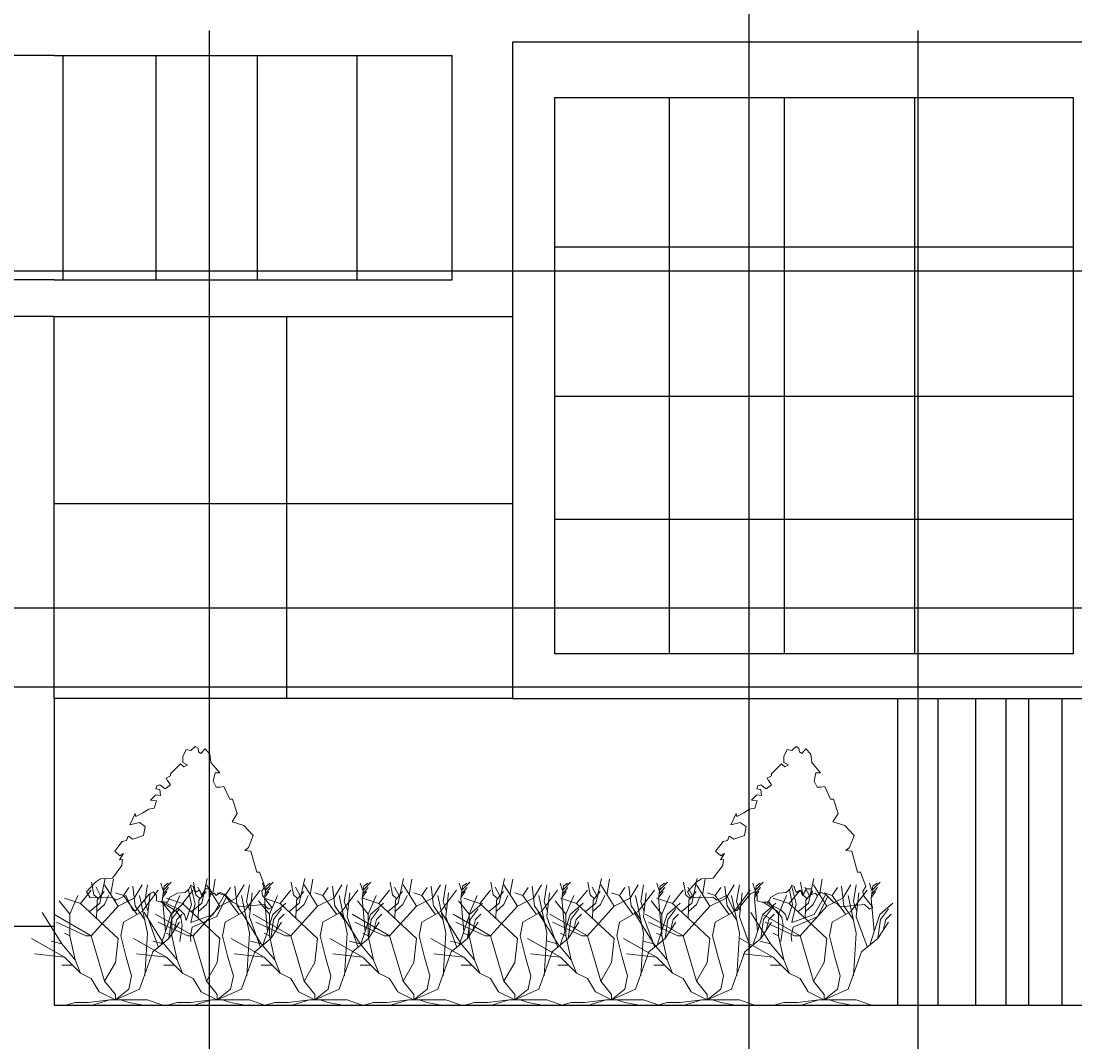
# Model space of a CAD drawing. Units: inches. Extents: x -117 to 121, y -77 to 40.
# Tile 22 of 45: x 3 to 28, y -32 to -8. Entities that reach past the tile are written whole.
import ezdxf

# ---------------------------------------------------------------- set-up
doc = ezdxf.new("R2010")
doc.units = ezdxf.units.IN
doc.header["$MEASUREMENT"] = 0
for name, color, linetype, lineweight in [('A-ANNO-DIMS', 2, 'Continuous', 18), ('A-ELEV', 7, 'Continuous', 25), ('L-PLNT', 3, 'Continuous', 13)]:
    doc.layers.add(name, color=color, linetype=linetype, lineweight=lineweight)
doc.styles.get("Standard").update_dxf_attribs({"font": 'arial.ttf'})
doc.dimstyles.get("Standard").update_dxf_attribs({"dimtxt": 0.18, "dimasz": 0.18, "dimexe": 0.18, "dimexo": 0.0625, "dimgap": 0.09, "dimtad": 0, "dimtih": 1, "dimtoh": 1, "dimdec": 4, "dimzin": 0, "dimdsep": 46, "dimtxsty": 'Standard', "dimcen": 0.09, "dimadec": 0, "dimazin": 0, "dimtfac": 1, "dimtdec": 4, "dimtofl": 0, "dimtmove": 0, "dimatfit": 3, "dimfxl": 1, "dimtolj": 1, "dimtzin": 0, "dimarcsym": 0})

# ---------------------------------------------------------------- blocks, each defined once
blk = doc.blocks.new('*U3')
for p, q in [((-11.433, 18.289), (-10.457, 22.749)), ((-12.471, 19.775), (-12.898, 22.044)), ((-11.28, 19.619), (-12.104, 21.184)), ((-8.16, 17.76), (-10.56, 21.6)), ((-9.48, 19.775), (-8.992, 22.592)), ((-7.2, 19.68), (-6.24, 21.12)), ((-5.086, 17.741), (-5.513, 21.34)), ((-5.28, 19.2), (-3.84, 21.6)), ((-3.377, 18.602), (-2.888, 21.575)), ((-0.508, 21.888), (-0.081, 20.558)), ((-0.203, 19.149), (0.102, 21.34)), ((-0.02, 20.01), (0.896, 21.105)), ((0.041, 20.714), (1.384, 22.044)), ((0.102, 21.34), (0.835, 21.888)), ((-14.88, 18.24), (-17.76, 19.2)), ((-16.8, 16.32), (-15.36, 19.68)), ((-14.88, 18.24), (-12.96, 20.64)), ((-11.677, 19.071), (-12.471, 19.775)), ((-11.921, 18.836), (-10.64, 20.401)), ((-10.579, 18.054), (-9.846, 19.697)), ((-7.2, 19.68), (-8.64, 20.16)), ((-8.16, 17.76), (-5.28, 19.2)), ((-4.8, 16.32), (-7.2, 19.68)), ((-2.88, 12.96), (-4.32, 19.68)), ((-3.84, 16.8), (-0.96, 20.64)), ((-2.88, 15.84), (-2.4, 20.16)), ((0.346, 13.203), (-0.203, 19.149)), ((-0.142, 19.384), (0.59, 20.401)), ((-16.8, 16.32), (-18.72, 18.72)), ((-8.16, 12), (-14.88, 18.24)), ((-13.325, 16.724), (-11.433, 18.289)), ((-12.96, 12.48), (-8.16, 17.76)), ((-12.043, 15.628), (-11.921, 18.836)), ((-11.982, 16.802), (-10.579, 18.054)), ((-3.377, 15.315), (-5.086, 17.819)), ((-2.766, 16.802), (-3.377, 18.602)), ((1.323, 16.254), (3.642, 18.289)), ((1.44, 15.36), (2.88, 17.28)), ((-18.24, 11.04), (-21.755, 16.655)), ((-12.96, 12.48), (-19.68, 16.32)), ((-16.8, 12.48), (-16.8, 16.32)), ((-7.2, 14.88), (-3.84, 16.8)), ((-0.96, 10.56), (-2.88, 15.84)), ((0.346, 13.203), (1.323, 16.254)), ((0.96, 12), (1.44, 15.36)), ((1.92, 13.44), (2.4, 15.36)), ((2.4, 15.36), (3.36, 16.32)), ((-13.92, 12.48), (-19.2, 14.88)), ((-7.68, 12.48), (-7.2, 14.88)), ((0.96, 12), (2.88, 14.88)), ((-17.76, 8.64), (-23.663, 11.961)), ((-18.24, 11.04), (-20.16, 11.52)), ((-16.8, 12.48), (-17.76, 12.96)), ((-15.84, 8.16), (-16.8, 12.48)), ((-12.96, 12.48), (-13.92, 12.48)), ((-10.56, 4.32), (-12.96, 12.48)), ((-8.64, 7.68), (-8.16, 12)), ((-6.72, 8.64), (-7.68, 12.48)), ((-3.36, 5.28), (-2.88, 12.96)), ((-1.92, 9.6), (0.96, 12)), ((-0.48, 10.8), (0.346, 13.203)), ((-15.84, 8.16), (-18.24, 11.04)), ((-4.32, 2.88), (-1.92, 9.6)), ((-17.76, 8.64), (-23.128, 9.222)), ((-14.88, 5.76), (-17.76, 8.64)), ((-14.88, 5.76), (-15.84, 8.16)), ((-10.56, 4.32), (-8.64, 7.68)), ((-5.76, 5.28), (-6.72, 8.64)), ((-16.32, 7.2), (-18.24, 7.2)), ((-12.96, 4.8), (-14.88, 5.76)), ((-11.52, 2.4), (-12.96, 4.8)), ((-8.64, 1.92), (-10.56, 4.32)), ((-6.24, 2.88), (-5.76, 5.28)), ((-8.64, 0.96), (-11.52, 2.4)), ((-8.64, 0.96), (-4.32, 2.88)), ((-8.64, 0.96), (-6.24, 2.88)), ((-8.64, 0.96), (-8.64, 1.92)), ((-15.84, 0.48), (-17.76, 0)), ((-13.44, 0.48), (-15.84, 0.48)), ((-9.6, 0.96), (-13.44, 0.48)), ((-9.6, 0.96), (-12.96, 0)), ((-9.6, 0.96), (-7.68, 0.96)), ((-8.64, 0.96), (-2.88, 0.96)), ((-7.68, 0.96), (-6.24, 0.48)), ((-6.24, 0.48), (-3.36, 0)), ((-2.88, 0.96), (0, 0))]:
    blk.add_line(p, q)
blk = doc.blocks.new('*U4')
for points in [[(22.0124, 137.721), (18.5475, 141.5624), (15.5282, 138.2446), (13.8028, 139.3505), (13.3714, 142.1153), (11.2148, 143.2214), (8.1954, 140.4564), (4.7447, 141.0094), (2.1567, 136.0326), (2.1567, 131.6088), (5.6074, 129.9499), (3.0193, 128.2909), (0.4313, 130.5029), (-6.9015, 123.3141), (-6.9015, 121.6552), (-9.9208, 119.9963), (-9.0581, 118.3373), (-6.9015, 115.0195), (-10.7835, 112.2546), (-14.6656, 115.0195), (-16.8222, 114.4665), (-17.6849, 112.2546), (-14.6656, 111.7016), (-14.2342, 107.2778), (-17.6065, 107.8307), (-21.5669, 103.9599), (-17.2536, 103.4069), (-18.9789, 97.8771), (-22.8609, 97.3241), (-27.1743, 94.5593), (-32.3504, 91.7944), (-32.7817, 94.0063), (-36.6638, 85.7116), (-29.7624, 87.3705), (-25.449, 84.6056), (-26.743, 77.9699), (-34.507, 75.205), (-37.9578, 77.4169), (-39.2518, 74.099), (-42.2711, 73.5461), (-44.8592, 70.2282), (-47.8786, 66.3574), (-43.9965, 63.0395), (-41.4085, 64.6985), (-44.3346, 59.8898), (-42.2089, 60.1377), (-42.5159, 55.7849), (-49.6039, 46.4502), (-58.2307, 45.8972), (-62.1127, 43.6853), (-68.5828, 36.4966), (-65.9947, 32.0727), (-50.0352, 32.6257), (-47.0159, 30.4138), (-39.6831, 33.7317), (-34.507, 22.6721), (-32.3504, 22.6721), (-22.4296, 34.8376), (-19.4102, 36.4966), (-17.2536, 33.7317), (-17.2536, 29.8608), (-13.8028, 28.7549), (-9.0581, 28.7549), (-7.3328, 32.6257), (-1.7254, 35.3906), (3.8821, 35.9436), (6.4701, 38.1555), (6.9014, 38.7085), (8.1954, 41.4734), (9.9208, 40.3674), (11.2148, 35.9436), (14.2341, 37.6025), (15.0968, 36.4966), (15.9595, 33.7317), (18.9789, 38.7085), (21.9982, 38.7085), (23.2922, 36.4966), (21.9982, 34.2847), (25.4489, 35.3906), (26.743, 33.7317), (29.7623, 35.9436), (32.7817, 34.8376), (38.8204, 28.7549), (41.4084, 27.6489), (43.5651, 25.437), (61.6813, 27.0959), (65.132, 23.7781), (67.7201, 24.884), (60.8186, 33.7317), (60.3873, 37.0495), (62.544, 40.3674), (58.662, 50.874), (56.5053, 50.874), (52.1919, 66.3574), (47.8785, 66.9103), (50.4665, 69.1222), (53.9172, 77.9699), (47.0158, 85.1586), (38.3891, 87.9235), (42.2711, 94.0063)], [(42.2711, 94.0063), (38.8204, 104.5129), (36.6637, 104.5129), (32.3503, 113.9135), (29.7623, 113.3605), (26.743, 113.3605), (24.5862, 117.7844), (25.8802, 123.8671), (29.331, 123.8671), (22.8609, 131.6088), (21.9982, 137.6916)], [(8.1954, 40.3674), (11.2148, 27.6489), (8.1954, 13.8245), (24.5862, 19.9072), (32.7817, 34.2847)], [(-9.9208, 28.2019), (0, 23.2251), (3.4507, 19.9072), (4.7447, 15.4834), (8.6267, 27.0959), (6.4701, 37.6025)], [(34.5071, 33.1787), (27.1743, 18.2483), (9.0581, 10.5066), (7.7641, 3.8708), (8.1954, 0)], [(-12.9401, 28.7549), (-2.588, 22.1191), (0.8626, 17.6953), (1.7253, 11.6125), (0, 0)]]:
    blk.add_lwpolyline(points)
blk = doc.blocks.new('*D32')
at = {"layer": 'A-ANNO-DIMS', "color": 0, "lineweight": -2, "transparency": 16777216}
for p, q in [((-3.85, -45.55), (-3.85, 38.61)), ((20.293, -45.55), (20.293, 38.61)), ((-3.67, 38.43), (7.757, 38.43)), ((20.113, 38.43), (8.686, 38.43))]:
    blk.add_line(p, q, dxfattribs=at)
at = {"layer": 'A-ANNO-DIMS', "color": 0, "transparency": 16777216}
for points in [[(-3.67, 38.46), (-3.67, 38.4), (-3.85, 38.43)], [(20.113, 38.46), (20.113, 38.4), (20.293, 38.43)]]:
    blk.add_solid(points, dxfattribs=at)
at = {"layer": 'Defpoints', "color": 0, "transparency": 16777216}
for p in [(20.293, 38.43), (-3.85, -45.613), (20.293, -45.613)]:
    blk.add_point(p, dxfattribs=at)
at = {"layer": 'A-ANNO-DIMS', "color": 0, "transparency": 16777216, "insert": (8.222, 38.43), "char_height": 0.18, "attachment_point": 5}
blk.add_mtext('\\A1;24.142', dxfattribs=at)
blk = doc.blocks.new('*D49')
at = {"layer": 'A-ANNO-DIMS', "color": 0, "lineweight": -2, "transparency": 16777216}
for p, q in [((-45.422, -23.501), (120.84, -23.501)), ((120.66, -23.681), (120.66, -31.426)), ((120.66, -39.536), (120.66, -31.79)), ((-45.471, -39.716), (120.84, -39.716))]:
    blk.add_line(p, q, dxfattribs=at)
at = {"layer": 'A-ANNO-DIMS', "color": 0, "transparency": 16777216}
for points in [[(120.63, -23.681), (120.69, -23.681), (120.66, -23.501)], [(120.63, -39.536), (120.69, -39.536), (120.66, -39.716)]]:
    blk.add_solid(points, dxfattribs=at)
at = {"layer": 'Defpoints', "color": 0, "transparency": 16777216}
for p in [(-45.485, -23.501), (120.66, -23.501), (-45.533, -39.716)]:
    blk.add_point(p, dxfattribs=at)
at = {"layer": 'A-ANNO-DIMS', "color": 0, "transparency": 16777216, "insert": (120.66, -31.608), "char_height": 0.18, "attachment_point": 5}
blk.add_mtext('\\A1;16.215', dxfattribs=at)
blk = doc.blocks.new('*D50')
at = {"layer": 'A-ANNO-DIMS', "color": 0, "lineweight": -2, "transparency": 16777216}
for p, q in [((-47.458, -13.74), (120.84, -13.74)), ((120.66, -13.92), (120.66, -17.512)), ((120.66, -21.468), (120.66, -17.876)), ((-47.458, -21.648), (120.84, -21.648))]:
    blk.add_line(p, q, dxfattribs=at)
at = {"layer": 'A-ANNO-DIMS', "color": 0, "transparency": 16777216}
for points in [[(120.63, -13.92), (120.69, -13.92), (120.66, -13.74)], [(120.63, -21.468), (120.69, -21.468), (120.66, -21.648)]]:
    blk.add_solid(points, dxfattribs=at)
at = {"layer": 'Defpoints', "color": 0, "transparency": 16777216}
for p in [(-47.521, -13.74), (120.66, -13.74), (-47.521, -21.648)]:
    blk.add_point(p, dxfattribs=at)
at = {"layer": 'A-ANNO-DIMS', "color": 0, "transparency": 16777216, "insert": (120.66, -17.694), "char_height": 0.18, "attachment_point": 5}
blk.add_mtext('\\A1;7.908', dxfattribs=at)
blk = doc.blocks.new('*D56')
at = {"layer": 'A-ANNO-DIMS', "color": 0, "lineweight": -2, "transparency": 16777216}
for p, q in [((-14.23, -7.853), (-14.23, -77.193)), ((7.628, -8.105), (7.628, -77.193)), ((-14.05, -77.013), (-3.766, -77.013)), ((7.448, -77.013), (-2.835, -77.013))]:
    blk.add_line(p, q, dxfattribs=at)
at = {"layer": 'A-ANNO-DIMS', "color": 0, "transparency": 16777216}
for points in [[(-14.05, -76.983), (-14.05, -77.043), (-14.23, -77.013)], [(7.448, -76.983), (7.448, -77.043), (7.628, -77.013)]]:
    blk.add_solid(points, dxfattribs=at)
at = {"layer": 'Defpoints', "color": 0, "transparency": 16777216}
for p in [(-14.23, -7.791), (7.628, -8.042), (7.628, -77.013)]:
    blk.add_point(p, dxfattribs=at)
at = {"layer": 'A-ANNO-DIMS', "color": 0, "transparency": 16777216, "insert": (-3.301, -77.013), "char_height": 0.18, "attachment_point": 5}
blk.add_mtext('\\A1;21.858', dxfattribs=at)
blk = doc.blocks.new('*D57')
at = {"layer": 'A-ANNO-DIMS', "color": 0, "lineweight": -2, "transparency": 16777216}
for p, q in [((7.628, -8.105), (7.628, -77.193)), ((24.248, -8.105), (24.248, -77.193)), ((7.808, -77.013), (15.483, -77.013)), ((24.068, -77.013), (16.393, -77.013))]:
    blk.add_line(p, q, dxfattribs=at)
at = {"layer": 'A-ANNO-DIMS', "color": 0, "transparency": 16777216}
for points in [[(7.808, -76.983), (7.808, -77.043), (7.628, -77.013)], [(24.068, -76.983), (24.068, -77.043), (24.248, -77.013)]]:
    blk.add_solid(points, dxfattribs=at)
at = {"layer": 'Defpoints', "color": 0, "transparency": 16777216}
for p in [(7.628, -8.042), (24.248, -8.042), (24.248, -77.013)]:
    blk.add_point(p, dxfattribs=at)
at = {"layer": 'A-ANNO-DIMS', "color": 0, "transparency": 16777216, "insert": (15.938, -77.013), "char_height": 0.18, "attachment_point": 5}
blk.add_mtext('\\A1;16.620', dxfattribs=at)
blk = doc.blocks.new('*D58')
at = {"layer": 'A-ANNO-DIMS', "color": 0, "lineweight": -2, "transparency": 16777216}
for p, q in [((24.248, -8.105), (24.248, -77.193)), ((57.61, -7.947), (57.61, -77.193)), ((24.428, -77.013), (40.467, -77.013)), ((57.43, -77.013), (41.392, -77.013))]:
    blk.add_line(p, q, dxfattribs=at)
at = {"layer": 'A-ANNO-DIMS', "color": 0, "transparency": 16777216}
for points in [[(24.428, -76.983), (24.428, -77.043), (24.248, -77.013)], [(57.43, -76.983), (57.43, -77.043), (57.61, -77.013)]]:
    blk.add_solid(points, dxfattribs=at)
at = {"layer": 'Defpoints', "color": 0, "transparency": 16777216}
for p in [(57.61, -7.885), (24.248, -8.042), (57.61, -77.013)]:
    blk.add_point(p, dxfattribs=at)
at = {"layer": 'A-ANNO-DIMS', "color": 0, "transparency": 16777216, "insert": (40.929, -77.013), "char_height": 0.18, "attachment_point": 5}
blk.add_mtext('\\A1;33.362', dxfattribs=at)

msp = doc.modelspace()

# ---------------------------------------------------------------- linework, layer by layer
at = {"layer": 'A-ELEV'}
for p, q in [((29.012, -8.3785), (14.7397, -8.3785)), ((14.7397, -8.3785), (14.7397, -8.8134)), ((3.9947, -8.6912), (-13.7272, -8.6912)), ((3.9947, -8.6912), (13.3263, -8.6912)), ((4.2039, -13.9556), (4.2039, -8.6912)), ((6.3832, -13.9556), (6.3832, -8.6912)), ((8.7651, -13.9556), (8.7651, -8.6912)), ((11.0964, -13.9556), (11.0964, -8.6912)), ((13.3263, -13.9556), (13.3263, -8.6912)), ((14.7397, -8.8134), (14.7397, -23.7756)), ((15.7326, -9.6801), (27.8856, -9.6801)), ((15.7326, -22.7278), (15.7326, -9.6801)), ((18.419, -9.6801), (18.419, -22.7278)), ((21.1133, -9.6801), (21.1133, -22.7278)), ((24.1718, -9.6801), (24.1718, -22.7278)), ((27.8856, -9.6801), (27.8856, -22.7278)), ((15.7326, -13.1807), (27.8856, -13.1807)), ((3.9947, -13.9556), (-13.7272, -13.9556)), ((3.9947, -13.9556), (13.3263, -13.9556)), ((3.9947, -14.8161), (-13.7272, -14.8161)), ((3.9947, -23.7756), (3.9947, -14.8161)), ((3.9947, -14.8161), (14.7397, -14.8161)), ((9.4524, -23.7756), (9.4524, -14.8161)), ((15.7326, -16.6813), (27.8856, -16.6813)), ((3.9947, -19.2007), (14.7397, -19.2007)), ((15.7326, -19.5699), (27.8856, -19.5699)), ((27.8856, -22.7278), (15.7326, -22.7278)), ((22.0645, -22.7074), (22.0645, -22.7278)), ((22.8894, -22.7074), (22.8894, -22.7278)), ((23.7732, -22.7074), (23.7732, -22.7278)), ((24.7159, -22.7074), (24.7159, -22.7278)), ((25.5997, -22.7074), (25.5997, -22.7278)), ((26.312, -22.7074), (26.312, -22.7278)), ((26.8414, -22.7074), (26.8414, -22.7278)), ((27.6241, -22.7074), (27.6241, -22.7278)), ((14.7397, -23.7756), (3.9947, -23.7756)), ((3.9947, -23.7756), (3.9947, -30.968)), ((14.7397, -23.7756), (29.012, -23.7756)), ((23.7732, -23.7756), (23.7732, -30.968)), ((24.7159, -23.7756), (24.7159, -30.968)), ((25.5997, -23.7756), (25.5997, -30.968)), ((26.312, -23.7756), (26.312, -30.968)), ((26.8414, -23.7756), (26.8414, -30.968)), ((27.6241, -23.7756), (27.6241, -30.968)), ((-13.7272, -29.1126), (3.9947, -29.1126)), ((3.9947, -30.968), (21.9795, -30.968)), ((21.9795, -30.968), (38.5013, -30.968))]:
    msp.add_line(p, q, dxfattribs=at)

# ---------------------------------------------------------------- block references
at = {"layer": 'L-PLNT'}
for name, p, xscale, yscale, zscale in [('*U4', (6.9415, -29.4693), 0.0318946538926936, 0.0318946538926936, 0.0318946538926936), ('*U4', (21.0324, -29.4693), 0.0318946538926936, 0.0318946538926936, 0.0318946538926936), ('*U3', (6.5606, -30.9685), 0.1308970629423973, 0.1308970629423973, 0.1308970629423973), ('*U3', (8.9503, -30.9685), 0.1308970629423973, 0.1308970629423973, 0.1308970629423973), ('*U3', (11.2403, -30.9685), 0.1308970629423973, 0.1308970629423973, 0.1308970629423973), ('*U3', (13.5583, -30.9685), 0.1308970629423973, 0.1308970629423973, 0.1308970629423973), ('*U3', (15.924, -30.9685), 0.1308970629423973, 0.1308970629423973, 0.1308970629423973), ('*U3', (18.1942, -30.9685), 0.1308970629423973, 0.1308970629423973, 0.1308970629423973), ('*U3', (20.4405, -30.9685), 0.1308970629423973, 0.1308970629423973, 0.1308970629423973), ('*U3', (23.1804, -30.9685), 0.1308970629423973, 0.1308970629423973, 0.1308970629423973)]:
    msp.add_blockref(name, p, dxfattribs=dict(at, xscale=xscale, yscale=yscale, zscale=zscale))

# ---------------------------------------------------------------- dimensions: what is measured, and where the dimension line sits
at = {"layer": 'A-ANNO-DIMS'}
for base, p1, p2, picture, middle in [((20.2929, 38.4297), (-3.8495, -45.6125), (20.2929, -45.6125), '*D32', (8.2217, 38.4297)), ((7.6284, -77.0135), (-14.2298, -7.7907), (7.6284, -8.0421), '*D56', (-3.3007, -77.0135)), ((57.6104, -77.0135), (24.2481, -8.0421), (57.6104, -7.8846), '*D58', (40.9293, -77.0135)), ((24.2481, -77.0135), (7.6284, -8.0421), (24.2481, -8.0421), '*D57', (15.9383, -77.0135))]:
    dim = msp.add_linear_dim(base=base, p1=p1, p2=p2, dimstyle='Standard', override={"dimdec": 3, "dimlfac": 1, "dimrnd": 0, "dimzin": 0, "dimdsep": 46, "dimlunit": 2}, dxfattribs=at)
    dim.commit()
    dim.dimension.update_dxf_attribs({"geometry": picture, "text_midpoint": middle})
for base, p1, p2, picture, middle in [((120.6602, -13.74), (-47.5206, -21.6476), (-47.5206, -13.74), '*D50', (120.6602, -17.6938)), ((120.6602, -23.5007), (-45.5331, -39.716), (-45.4848, -23.5007), '*D49', (120.6602, -31.6083))]:
    dim = msp.add_linear_dim(base=base, p1=p1, p2=p2, angle=90, dimstyle='Standard', override={"dimdec": 3, "dimlfac": 1, "dimrnd": 0, "dimzin": 0, "dimdsep": 46, "dimlunit": 2}, dxfattribs=at)
    dim.commit()
    dim.dimension.update_dxf_attribs({"geometry": picture, "text_midpoint": middle})

doc.saveas('drawing.dxf')
